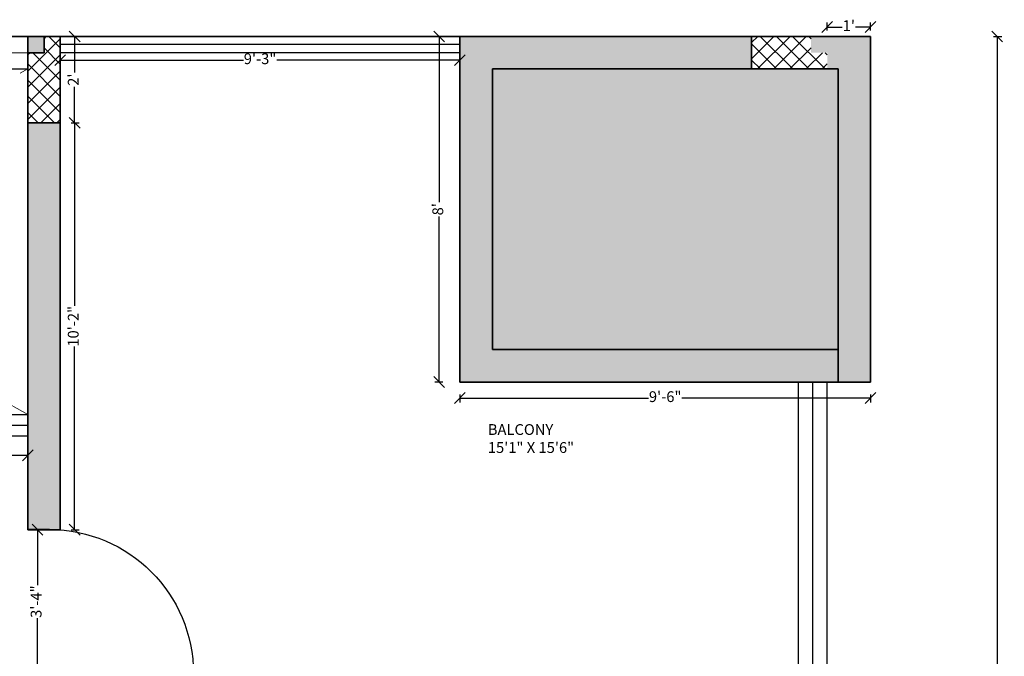
# Model space of a CAD drawing. Units: inches. Extents: x 1365 to 2091, y 1589 to 2091.
# Tile 8 of 8: x 1818 to 2091, y 1891 to 2068. Entities that reach past the tile are written whole.
import ezdxf

# ---------------------------------------------------------------- set-up
doc = ezdxf.new("R2010")
doc.units = ezdxf.units.IN
doc.linetypes.add('ACAD_ISO02W100', pattern=[15, 12, -3])
for name, color, linetype, lineweight in [('A-ANNO-DIMS', 2, 'Continuous', 18), ('A-AREA-IDEN', 7, 'Continuous', 18), ('A-COLS', 7, 'Continuous', 35), ('A-COLS-MARK-PATT', 114, 'Continuous', 13), ('A-COLS-PATT', 1, 'Continuous', 13), ('A-DOOR', 4, 'Continuous', 25), ('A-FLOR-HRAL', 7, 'Continuous', 25), ('A-FLOR-OPEN', 7, 'Continuous', 25), ('A-FLOR-OPEN-HIDN', 1, 'ACAD_ISO02W100', 18), ('A-FLOR-PATT', 143, 'Continuous', 13), ('A-WALL', 7, 'Continuous', 35), ('A-WALL-PATT', 253, 'Continuous', 13)]:
    doc.layers.add(name, color=color, linetype=linetype, lineweight=lineweight)
doc.styles.get("Standard").update_dxf_attribs({"font": 'arial.ttf'})
doc.dimstyles.new('ISO-25', dxfattribs={"dimtxt": 3, "dimasz": 3, "dimexe": 1.25, "dimexo": 0.625, "dimtad": 0, "dimlunit": 4, "dimtxsty": 'Standard', "dimblk": 'OBLIQUE', "dimcen": 2.5, "dimclrd": 254, "dimclre": 254, "dimclrt": 1, "dimadec": 0, "dimazin": 0, "dimtfac": 1, "dimtmove": 0, "dimatfit": 3, "dimfxl": 1, "dimfxlon": 1, "dimfrac": 1, "dimarcsym": 0})

# ---------------------------------------------------------------- blocks, each defined once
blk = doc.blocks.new('*U5')
for p, q in [((0, 0), (0, -6)), ((40, 0), (40, -6))]:
    blk.add_line(p, q)
blk.add_lwpolyline([(0, 0), (0, 40), (1.75, 40), (1.75, 0)], close=True)
blk.add_arc((0, 0), 40, 0, 90)
blk = doc.blocks.new('_Oblique')
at = {"color": 0, "linetype": 'ByBlock', "lineweight": -2}
blk.add_line((-0.5, -0.5), (0.5, 0.5), dxfattribs=at)
blk = doc.blocks.new('*D15')
at = {"layer": 'A-ANNO-DIMS', "color": 0, "lineweight": -2, "transparency": 16777216}
for p, q in [((1828.75, 2057.29), (1828.75, 2055.04)), ((1828.75, 2056.29), (1879.64, 2056.29)), ((1939.75, 2056.29), (1888.87, 2056.29)), ((1939.75, 2057.29), (1939.75, 2055.04))]:
    blk.add_line(p, q, dxfattribs=at)
at = {"layer": 'Defpoints', "color": 0, "transparency": 16777216}
for p in [(1828.75, 2058.36), (1939.75, 2058.36), (1939.75, 2056.29)]:
    blk.add_point(p, dxfattribs=at)
at = {"layer": 'A-ANNO-DIMS', "color": 0, "lineweight": -2, "transparency": 16777216, "xscale": 3, "yscale": 3, "zscale": 3, "rotation": 180}
blk.add_blockref('_Oblique', (1828.75, 2056.29), dxfattribs=at)
at = {"layer": 'A-ANNO-DIMS', "color": 0, "lineweight": -2, "transparency": 16777216, "xscale": 3, "yscale": 3, "zscale": 3}
blk.add_blockref('_Oblique', (1939.75, 2056.29), dxfattribs=at)
at = {"layer": 'A-ANNO-DIMS', "color": 0, "transparency": 16777216, "insert": (1884.25, 2056.29), "char_height": 3, "attachment_point": 5}
blk.add_mtext('9\'-3"', dxfattribs=at)
blk = doc.blocks.new('*D87')
at = {"layer": 'A-ANNO-DIMS', "color": 0, "lineweight": -2, "transparency": 16777216}
for p, q in [((1934.99, 2062.86), (1932.74, 2062.86)), ((1933.99, 2062.86), (1933.99, 2016.86)), ((1933.99, 1966.86), (1933.99, 2012.85)), ((1934.99, 1966.86), (1932.74, 1966.86))]:
    blk.add_line(p, q, dxfattribs=at)
at = {"layer": 'Defpoints', "color": 0, "transparency": 16777216}
for p in [(1939.75, 2062.86), (1933.99, 1966.86), (1939.75, 1966.86)]:
    blk.add_point(p, dxfattribs=at)
at = {"layer": 'A-ANNO-DIMS', "color": 0, "lineweight": -2, "transparency": 16777216, "xscale": 3, "yscale": 3, "zscale": 3}
for p, rotation in [((1933.99, 2062.86), 90), ((1933.99, 1966.86), 270)]:
    blk.add_blockref('_Oblique', p, dxfattribs=dict(at, rotation=rotation))
at = {"layer": 'A-ANNO-DIMS', "color": 0, "transparency": 16777216, "insert": (1933.99, 2014.86), "char_height": 3, "attachment_point": 5, "rotation": 90}
blk.add_mtext("8'", dxfattribs=at)
blk = doc.blocks.new('*D88')
at = {"layer": 'A-ANNO-DIMS', "color": 0, "lineweight": -2, "transparency": 16777216}
for p, q in [((1939.75, 1963.4), (1939.75, 1961.15)), ((2053.75, 1963.4), (2053.75, 1961.15)), ((1939.75, 1962.4), (1992.14, 1962.4)), ((2053.75, 1962.4), (2001.37, 1962.4))]:
    blk.add_line(p, q, dxfattribs=at)
at = {"layer": 'Defpoints', "color": 0, "transparency": 16777216}
for p in [(1939.75, 1967.58), (2053.75, 1966.86), (2053.75, 1962.4)]:
    blk.add_point(p, dxfattribs=at)
at = {"layer": 'A-ANNO-DIMS', "color": 0, "lineweight": -2, "transparency": 16777216, "xscale": 3, "yscale": 3, "zscale": 3, "rotation": 180}
blk.add_blockref('_Oblique', (1939.75, 1962.4), dxfattribs=at)
at = {"layer": 'A-ANNO-DIMS', "color": 0, "lineweight": -2, "transparency": 16777216, "xscale": 3, "yscale": 3, "zscale": 3}
blk.add_blockref('_Oblique', (2053.75, 1962.4), dxfattribs=at)
at = {"layer": 'A-ANNO-DIMS', "color": 0, "transparency": 16777216, "insert": (1996.75, 1962.4), "char_height": 3, "attachment_point": 5}
blk.add_mtext('9\'-6"', dxfattribs=at)
blk = doc.blocks.new('*D89')
at = {"layer": 'A-ANNO-DIMS', "color": 0, "lineweight": -2, "transparency": 16777216}
for p, q in [((2041.75, 2064.49), (2041.75, 2066.74)), ((2041.75, 2065.49), (2045.89, 2065.49)), ((2053.75, 2065.49), (2049.62, 2065.49)), ((2053.75, 2064.49), (2053.75, 2066.74))]:
    blk.add_line(p, q, dxfattribs=at)
at = {"layer": 'Defpoints', "color": 0, "transparency": 16777216}
for p in [(2041.75, 2065.49), (2041.75, 2062.86), (2053.75, 2062.86)]:
    blk.add_point(p, dxfattribs=at)
at = {"layer": 'A-ANNO-DIMS', "color": 0, "lineweight": -2, "transparency": 16777216, "xscale": 3, "yscale": 3, "zscale": 3, "rotation": 180}
blk.add_blockref('_Oblique', (2041.75, 2065.49), dxfattribs=at)
at = {"layer": 'A-ANNO-DIMS', "color": 0, "lineweight": -2, "transparency": 16777216, "xscale": 3, "yscale": 3, "zscale": 3}
blk.add_blockref('_Oblique', (2053.75, 2065.49), dxfattribs=at)
at = {"layer": 'A-ANNO-DIMS', "color": 0, "transparency": 16777216, "insert": (2047.75, 2065.49), "char_height": 3, "attachment_point": 5}
blk.add_mtext("1'", dxfattribs=at)
blk = doc.blocks.new('*D90')
at = {"layer": 'A-ANNO-DIMS', "color": 0, "lineweight": -2, "transparency": 16777216}
for p, q in [((1831.76, 2062.86), (1834.01, 2062.86)), ((1832.76, 2062.86), (1832.76, 2052.89)), ((1832.76, 2038.86), (1832.76, 2048.83)), ((1831.76, 2038.86), (1834.01, 2038.86))]:
    blk.add_line(p, q, dxfattribs=at)
at = {"layer": 'Defpoints', "color": 0, "transparency": 16777216}
for p in [(1828.75, 2062.86), (1828.75, 2038.86), (1832.76, 2038.86)]:
    blk.add_point(p, dxfattribs=at)
at = {"layer": 'A-ANNO-DIMS', "color": 0, "lineweight": -2, "transparency": 16777216, "xscale": 3, "yscale": 3, "zscale": 3}
for p, rotation in [((1832.76, 2062.86), 90), ((1832.76, 2038.86), 270)]:
    blk.add_blockref('_Oblique', p, dxfattribs=dict(at, rotation=rotation))
at = {"layer": 'A-ANNO-DIMS', "color": 0, "transparency": 16777216, "insert": (1832.76, 2050.86), "char_height": 3, "attachment_point": 5, "rotation": 90}
blk.add_mtext("2'", dxfattribs=at)
blk = doc.blocks.new('*D91')
at = {"layer": 'A-ANNO-DIMS', "color": 0, "lineweight": -2, "transparency": 16777216}
for p, q in [((1831.76, 2038.86), (1834.01, 2038.86)), ((1832.76, 2038.86), (1832.76, 1987.98)), ((1832.76, 1925.83), (1832.76, 1976.71)), ((1831.76, 1925.83), (1834.01, 1925.83))]:
    blk.add_line(p, q, dxfattribs=at)
at = {"layer": 'Defpoints', "color": 0, "transparency": 16777216}
for p in [(1828.75, 2038.86), (1828.75, 1925.83), (1832.76, 1925.83)]:
    blk.add_point(p, dxfattribs=at)
at = {"layer": 'A-ANNO-DIMS', "color": 0, "lineweight": -2, "transparency": 16777216, "xscale": 3, "yscale": 3, "zscale": 3}
for p, rotation in [((1832.76, 2038.86), 90), ((1832.76, 1925.83), 270)]:
    blk.add_blockref('_Oblique', p, dxfattribs=dict(at, rotation=rotation))
at = {"layer": 'A-ANNO-DIMS', "color": 0, "transparency": 16777216, "insert": (1832.76, 1982.34), "char_height": 3, "attachment_point": 5, "rotation": 90}
blk.add_mtext('10\'-2"', dxfattribs=at)
blk = doc.blocks.new('*D92')
at = {"layer": 'A-ANNO-DIMS', "color": 0, "lineweight": -2, "transparency": 16777216}
for p, q in [((1821.45, 1925.83), (1823.7, 1925.83)), ((1822.45, 1925.83), (1822.45, 1910.45)), ((1822.45, 1885.86), (1822.45, 1901.23)), ((1821.45, 1885.86), (1823.7, 1885.86))]:
    blk.add_line(p, q, dxfattribs=at)
at = {"layer": 'Defpoints', "color": 0, "transparency": 16777216}
for p in [(1819.75, 1925.83), (1819.75, 1885.86), (1822.45, 1885.86)]:
    blk.add_point(p, dxfattribs=at)
at = {"layer": 'A-ANNO-DIMS', "color": 0, "lineweight": -2, "transparency": 16777216, "xscale": 3, "yscale": 3, "zscale": 3}
for p, rotation in [((1822.45, 1925.83), 90), ((1822.45, 1885.86), 270)]:
    blk.add_blockref('_Oblique', p, dxfattribs=dict(at, rotation=rotation))
at = {"layer": 'A-ANNO-DIMS', "color": 0, "transparency": 16777216, "insert": (1822.45, 1905.84), "char_height": 3, "attachment_point": 5, "rotation": 90}
blk.add_mtext('3\'-4"', dxfattribs=at)
blk = doc.blocks.new('*D93')
at = {"layer": 'A-ANNO-DIMS', "color": 0, "lineweight": -2, "transparency": 16777216}
for p, q in [((1647.25, 1947.47), (1647.25, 1945.22)), ((1819.75, 1947.47), (1819.75, 1945.22)), ((1647.25, 1946.47), (1725.72, 1946.47)), ((1819.75, 1946.47), (1741.29, 1946.47))]:
    blk.add_line(p, q, dxfattribs=at)
at = {"layer": 'Defpoints', "color": 0, "transparency": 16777216}
for p in [(1647.25, 1951.86), (1819.75, 1951.86), (1819.75, 1946.47)]:
    blk.add_point(p, dxfattribs=at)
at = {"layer": 'A-ANNO-DIMS', "color": 0, "lineweight": -2, "transparency": 16777216, "xscale": 3, "yscale": 3, "zscale": 3, "rotation": 180}
blk.add_blockref('_Oblique', (1647.25, 1946.47), dxfattribs=at)
at = {"layer": 'A-ANNO-DIMS', "color": 0, "lineweight": -2, "transparency": 16777216, "xscale": 3, "yscale": 3, "zscale": 3}
blk.add_blockref('_Oblique', (1819.75, 1946.47), dxfattribs=at)
at = {"layer": 'A-ANNO-DIMS', "color": 0, "transparency": 16777216, "insert": (1733.5, 1946.47), "char_height": 3, "attachment_point": 5}
blk.add_mtext('14\'-4{\\H1x;\\S1#2;}"', dxfattribs=at)
blk = doc.blocks.new('*D123')
at = {"layer": 'A-ANNO-DIMS', "color": 254, "lineweight": -2, "transparency": 16777216}
for p, q in [((2087.95, 2062.86), (2090.2, 2062.86)), ((2088.95, 2062.86), (2088.95, 1858.63)), ((2088.95, 1642.86), (2088.95, 1847.08)), ((2087.95, 1642.86), (2090.2, 1642.86))]:
    blk.add_line(p, q, dxfattribs=at)
at = {"layer": 'Defpoints', "color": 0, "transparency": 16777216}
for p in [(2053.75, 2062.86), (2088.95, 2062.86), (2053.75, 1642.86)]:
    blk.add_point(p, dxfattribs=at)
at = {"layer": 'A-ANNO-DIMS', "color": 254, "lineweight": -2, "transparency": 16777216, "xscale": 3, "yscale": 3, "zscale": 3}
for p, rotation in [((2088.95, 2062.86), 90), ((2088.95, 1642.86), 270)]:
    blk.add_blockref('_Oblique', p, dxfattribs=dict(at, rotation=rotation))
at = {"layer": 'A-ANNO-DIMS', "color": 1, "transparency": 16777216, "insert": (2088.95, 1852.86), "char_height": 3, "attachment_point": 5, "rotation": 90}
blk.add_mtext('35\'-0"', dxfattribs=at)

msp = doc.modelspace()

# ---------------------------------------------------------------- hatches: boundary and pattern name
at = {"layer": 'A-COLS-MARK-PATT'}
h = msp.add_hatch(color=256, dxfattribs=at)
h.dxf.hatch_style = 1
h.paths.add_polyline_path([(1398.254, 2062.858), (1393.754, 2062.858), (1393.754, 2058.358), (1398.254, 2058.358)])
h.paths.add_polyline_path([(1398.254, 1872.358), (1393.754, 1872.358), (1393.754, 1867.858), (1398.254, 1867.858)])
h.paths.add_polyline_path([(1398.254, 1807.858), (1393.754, 1807.858), (1393.754, 1803.358), (1398.254, 1803.358)])
h.paths.add_polyline_path([(1398.254, 1647.358), (1393.754, 1647.358), (1393.754, 1642.858), (1398.254, 1642.858)])
h.paths.add_polyline_path([(1638.254, 1647.358), (1633.754, 1647.358), (1633.754, 1642.858), (1638.254, 1642.858)])
h.paths.add_polyline_path([(1638.254, 1732.858), (1633.754, 1732.858), (1633.754, 1728.358), (1638.254, 1728.358)])
h.paths.add_polyline_path([(1647.254, 1876.858), (1642.754, 1876.858), (1642.754, 1872.358), (1647.254, 1872.358)])
h.paths.add_polyline_path([(1647.254, 1803.358), (1642.754, 1803.358), (1642.754, 1798.858), (1647.254, 1798.858)])
h.paths.add_polyline_path([(1647.254, 2062.858), (1642.754, 2062.858), (1642.754, 2058.358), (1647.254, 2058.358)])
h.paths.add_polyline_path([(1824.254, 2062.858), (1819.754, 2062.858), (1819.754, 2058.358), (1824.254, 2058.358)])
h.paths.add_polyline_path([(1824.254, 1885.858), (1819.754, 1885.858), (1819.754, 1881.358), (1824.254, 1881.358)])
h.paths.add_polyline_path([(1828.754, 1647.358), (1824.254, 1647.358), (1824.254, 1642.858), (1828.754, 1642.858)])
h.paths.add_polyline_path([(1948.754, 1647.358), (1944.254, 1647.358), (1944.254, 1642.858), (1948.754, 1642.858)])
h.paths.add_polyline_path([(2041.754, 1647.358), (2037.254, 1647.358), (2037.254, 1642.858), (2041.754, 1642.858)])
h.paths.add_polyline_path([(2041.754, 1885.858), (2037.254, 1885.858), (2037.254, 1881.358), (2041.754, 1881.358)])
h.paths.add_polyline_path([(2041.754, 2062.858), (2037.254, 2062.858), (2037.254, 2058.358), (2041.754, 2058.358)])
at = {"layer": 'A-COLS-PATT'}
h = msp.add_hatch(dxfattribs=at)
h.set_pattern_fill('ANSI37', color=256)
h.paths.add_polyline_path([(1642.754, 1803.358), (1647.254, 1803.358), (1647.254, 1807.858), (1629.254, 1807.858), (1629.254, 1798.858), (1633.754, 1798.858), (1642.754, 1798.858)])
h.paths.add_polyline_path([(1647.254, 1872.358), (1642.754, 1872.358), (1642.754, 1876.858), (1641.254, 1876.858), (1623.254, 1876.858), (1623.254, 1867.858), (1638.254, 1867.858), (1647.254, 1867.858)])
h.paths.add_polyline_path([(1647.254, 2058.358), (1642.754, 2058.358), (1642.754, 2062.858), (1638.254, 2062.858), (1638.254, 2053.858), (1647.254, 2053.858)])
h.paths.add_polyline_path([(1642.754, 2053.858), (1638.254, 2053.858), (1638.254, 2041.858), (1642.754, 2041.858)])
h.paths.add_polyline_path([(1647.254, 2053.858), (1642.754, 2053.858), (1642.754, 2041.858), (1647.254, 2041.858)])
h.paths.add_polyline_path([(1828.754, 2062.858), (1824.254, 2062.858), (1824.254, 2058.358), (1819.754, 2058.358), (1819.754, 2038.858), (1828.754, 2038.858)])
h.paths.add_polyline_path([(1839.254, 1885.858), (1825.754, 1885.858), (1824.254, 1885.858), (1824.254, 1881.358), (1819.754, 1881.358), (1819.754, 1876.858), (1839.254, 1876.858)])
h.paths.add_polyline_path([(2041.754, 1881.358), (2037.254, 1881.358), (2037.254, 1885.858), (2023.754, 1885.858), (2023.754, 1876.858), (2041.754, 1876.858)])
h.paths.add_polyline_path([(1828.754, 1666.858), (1819.754, 1666.858), (1819.754, 1642.858), (1824.254, 1642.858), (1824.254, 1647.358), (1828.754, 1647.358)])
h.paths.add_polyline_path([(1944.254, 1647.358), (1948.754, 1647.358), (1948.754, 1651.858), (1930.754, 1651.858), (1930.754, 1642.858), (1944.254, 1642.858)])
h.paths.add_polyline_path([(2037.254, 1647.358), (2041.754, 1647.358), (2041.754, 1651.858), (2023.754, 1651.858), (2023.754, 1642.858), (2037.254, 1642.858)])
h = msp.add_hatch(dxfattribs=at)
h.set_pattern_fill('ANSI37', color=256)
h.paths.add_polyline_path([(2037.254, 2062.858), (2020.754, 2062.858), (2020.754, 2053.858), (2041.754, 2053.858), (2041.754, 2058.358), (2037.254, 2058.358)])
at = {"layer": 'A-FLOR-PATT', "transparency": 33554544}
h = msp.add_hatch(color=256, dxfattribs=at)
h.dxf.hatch_style = 1
h.paths.add_polyline_path([(2044.754, 2053.858), (1948.754, 2053.858), (1948.754, 1975.858), (2044.754, 1975.858)])
at = {"layer": 'A-WALL-PATT'}
h = msp.add_hatch(color=256, dxfattribs=at)
h.dxf.hatch_style = 1
h.paths.add_polyline_path([(1638.254, 2053.858), (1638.254, 2062.858), (1617.254, 2062.858), (1617.254, 2053.858)])
h.paths.add_polyline_path([(1633.754, 1780.858), (1638.254, 1780.858), (1638.254, 1798.858), (1633.754, 1798.858)])
h.paths.add_polyline_path([(1828.754, 2038.858), (1819.754, 2038.858), (1819.754, 1925.829), (1828.754, 1925.829)])
h = msp.add_hatch(color=256, dxfattribs=at)
h.dxf.hatch_style = 1
h.paths.add_polyline_path([(2020.754, 2053.858), (2020.754, 2062.858), (1939.754, 2062.858), (1939.754, 1966.858), (2044.754, 1966.858), (2044.754, 1975.858), (1948.754, 1975.858), (1948.754, 2053.858)])
h = msp.add_hatch(color=256, dxfattribs=at)
h.dxf.hatch_style = 1
h.paths.add_polyline_path([(2044.754, 2062.858), (2041.754, 2062.858), (2041.754, 2053.858), (2044.754, 2053.858)])
h = msp.add_hatch(color=256, dxfattribs=at)
h.dxf.hatch_style = 1
h.paths.add_polyline_path([(2053.754, 2062.858), (2044.754, 2062.858), (2044.754, 1966.858), (2053.754, 1966.858)])

# ---------------------------------------------------------------- linework, layer by layer
at = {"layer": 'A-COLS'}
for p, q in [((1824.254, 2062.858), (1824.254, 2058.358)), ((2020.754, 2053.858), (2020.754, 2062.858)), ((1824.254, 2058.358), (1819.754, 2058.358)), ((1819.754, 2038.858), (1828.754, 2038.858))]:
    msp.add_line(p, q, dxfattribs=at)
at = {"layer": 'A-FLOR-HRAL'}
for p, q in [((1939.754, 2060.608), (1828.754, 2060.608)), ((1939.754, 2058.358), (1828.754, 2058.358)), ((2033.754, 1885.858), (2033.754, 1966.858)), ((2037.754, 1885.858), (2037.754, 1966.858)), ((2041.754, 1885.858), (2041.754, 1966.858)), ((1647.254, 1957.858), (1819.754, 1957.858)), ((1647.254, 1954.858), (1819.754, 1954.858)), ((1647.254, 1951.858), (1819.754, 1951.858))]:
    msp.add_line(p, q, dxfattribs=at)
at = {"layer": 'A-FLOR-OPEN'}
msp.add_line((1647.254, 2053.858), (1819.754, 2053.858), dxfattribs=at)
at = {"layer": 'A-FLOR-OPEN-HIDN'}
for p, q in [((1819.754, 2058.358), (1647.254, 2058.358)), ((1819.754, 1957.858), (1647.254, 2053.858)), ((1647.254, 1957.858), (1819.754, 2053.858))]:
    msp.add_line(p, q, dxfattribs=at)
at = {"layer": 'A-WALL'}
for p, q in [((1393.754, 2062.858), (2053.754, 2062.858)), ((1819.754, 1925.829), (1819.754, 2062.858)), ((1828.754, 2062.858), (1828.754, 2038.858)), ((1939.754, 1966.858), (1939.754, 2062.858)), ((2053.754, 2062.858), (2053.754, 1966.858)), ((1948.754, 1975.858), (1948.754, 2053.858)), ((1948.754, 2053.858), (2044.754, 2053.858)), ((2044.754, 2053.858), (2044.754, 1966.858)), ((1828.754, 2038.858), (1828.754, 1925.829)), ((2044.754, 1975.858), (1948.754, 1975.858)), ((2053.754, 1966.858), (1939.754, 1966.858)), ((1828.754, 1925.829), (1819.754, 1925.829))]:
    msp.add_line(p, q, dxfattribs=at)

# ---------------------------------------------------------------- block references
at = {"layer": 'A-DOOR', "xscale": -1, "rotation": 270}
msp.add_blockref('*U5', (1825.754, 1885.858), dxfattribs=at)

# ---------------------------------------------------------------- texts
at = {"layer": 'A-AREA-IDEN', "insert": (1947.499, 1955.157), "char_height": 3, "attachment_point": 1}
msp.add_mtext_dynamic_manual_height_columns('{BALCONY\\P15\'1" X 15\'6"}', width=33.58604, gutter_width=12.5, heights=[0], dxfattribs=at)

# ---------------------------------------------------------------- dimensions: what is measured, and where the dimension line sits
at = {"layer": 'A-ANNO-DIMS'}
for base, p1, p2, picture, middle in [((2041.754, 2065.485), (2053.754, 2062.858), (2041.754, 2062.858), '*D89', (2047.754, 2065.485)), ((1939.754, 2056.289), (1828.754, 2058.358), (1939.754, 2058.358), '*D15', (1884.254, 2056.289)), ((2053.754, 1962.402), (1939.754, 1967.577), (2053.754, 1966.858), '*D88', (1996.754, 1962.402)), ((1819.754, 1946.468), (1647.254, 1951.858), (1819.754, 1951.858), '*D93', (1733.504, 1946.468))]:
    dim = msp.add_linear_dim(base=base, p1=p1, p2=p2, dimstyle='ISO-25', override={"dimclrd": 0, "dimclre": 0, "dimclrt": 0}, dxfattribs=at)
    dim.commit()
    dim.dimension.update_dxf_attribs({"geometry": picture, "text_midpoint": middle})
for base, p1, p2, override, picture, middle in [((1832.759, 2038.858), (1828.754, 2062.858), (1828.754, 2038.858), {"dimclrd": 0, "dimclre": 0, "dimclrt": 0}, '*D90', (1832.759, 2050.858)), ((1933.994, 1966.858), (1939.754, 2062.858), (1939.754, 1966.858), {"dimclrd": 0, "dimclre": 0, "dimclrt": 0}, '*D87', (1933.994, 2014.858)), ((2088.954, 2062.858), (2053.754, 1642.858), (2053.754, 2062.858), {"dimdec": 1, "dimlfac": 1, "dimrnd": 0, "dimzin": 1, "dimdsep": 46, "dimlunit": 4, "dimfrac": 2}, '*D123', (2088.954, 1852.858)), ((1822.447, 1885.858), (1819.754, 1925.829), (1819.754, 1885.858), {"dimclrd": 0, "dimclre": 0, "dimclrt": 0}, '*D92', (1822.447, 1905.843))]:
    dim = msp.add_linear_dim(base=base, p1=p1, p2=p2, angle=90, dimstyle='ISO-25', override=override, dxfattribs=at)
    dim.commit()
    dim.dimension.update_dxf_attribs({"geometry": picture, "text_midpoint": middle})
dim = msp.add_linear_dim(base=(1832.759, 1925.829), p1=(1828.754, 2038.858), p2=(1828.754, 1925.829), angle=90, text='10\'-2"', dimstyle='ISO-25', override={"dimclrd": 0, "dimclre": 0, "dimclrt": 0, "dimtmove": 1}, dxfattribs=at)
dim.commit()
dim.dimension.update_dxf_attribs({"geometry": '*D91', "text_midpoint": (1832.759, 1982.343)})

doc.saveas('drawing.dxf')
